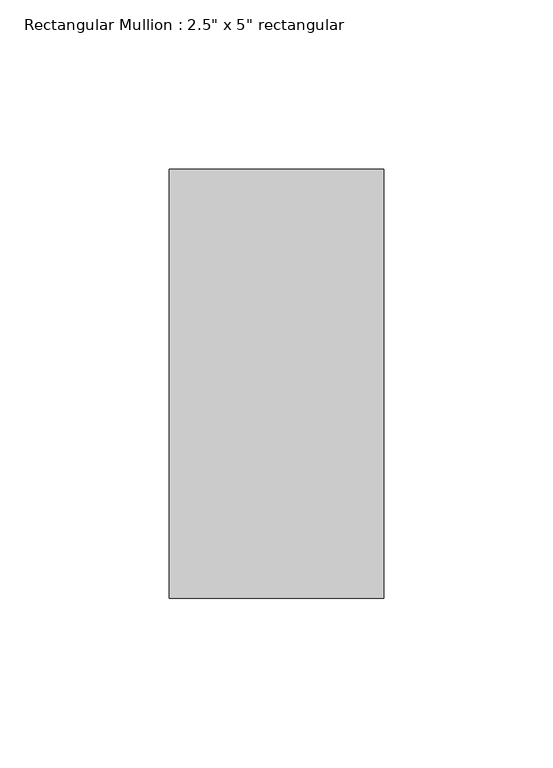
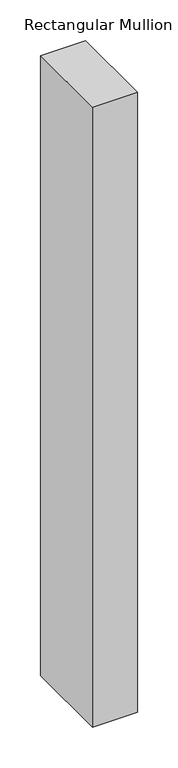
"""IFC4 building model written with IfcOpenShell, lengths in millimetres: member geometry."""

from ifc_helpers import new_model, si_unit, frame, origin, place, context, project, spatial, polyline, outline, extrude, source, transform, mapped, element, save


def member_f689fba6(model_context):
    return source(origin(), model_context, "Body", "SweptSolid", [
        extrude(outline(polyline([(0.0, 63.5), (0.0, -63.5), (-63.5, -63.5), (-63.5, 63.5), (0.0, 63.5)])), frame((0.0, 0.0, -927.1), z_axis=(0.0, 0.0, 1.0), x_axis=(1.0, 0.0, 0.0)), (0.0, 0.0, 1.0), 927.1),
    ])


if __name__ == "__main__":
    model = new_model("IFC4")
    model_context = context("Model", 3, world=origin())
    ifc_project = project(units=[si_unit("LENGTHUNIT", "METRE", prefix="MILLI")], contexts=[model_context])
    site = spatial("IfcSite", under=ifc_project)
    building = spatial("IfcBuilding", under=site)
    placement = place(None, origin())
    member_shape = member_f689fba6(model_context)
    element("IfcMember", 1, ObjectType="Rectangular Mullion : 2.5\" x 5\" rectangular", at=placement, inside=building, context=model_context, shape_type="MappedRepresentation", body=[
        mapped(member_shape, transform((0.0, 0.0, 0.0), x_axis=(1.0, 0.0, 0.0), y_axis=(0.0, 1.0, 0.0), z_axis=(0.0, 0.0, 1.0))),
    ])
    save(model, "model.ifc")

# Revit data of these elements
# Type "Rectangular Mullion : 2.5\" x 5\" rectangular"
#   built-in parameter 1007304 = 0.416667 (stored number, unit not read)
#   built-in parameter 1007301 = 0.104167 (stored number, unit not read)
#   built-in parameter 1007300 = 0.104167 (stored number, unit not read)
# Element 1 (IfcMember, "Rectangular Mullion : 2.5\" x 5\" rectangular")
#   Materials on its faces: "Aluminum"
# Materials
#   "Aluminum": class "Metal", colour RGB 247 247 247, transparency 0, Description = "Aluminum 6061", Cost = 0
